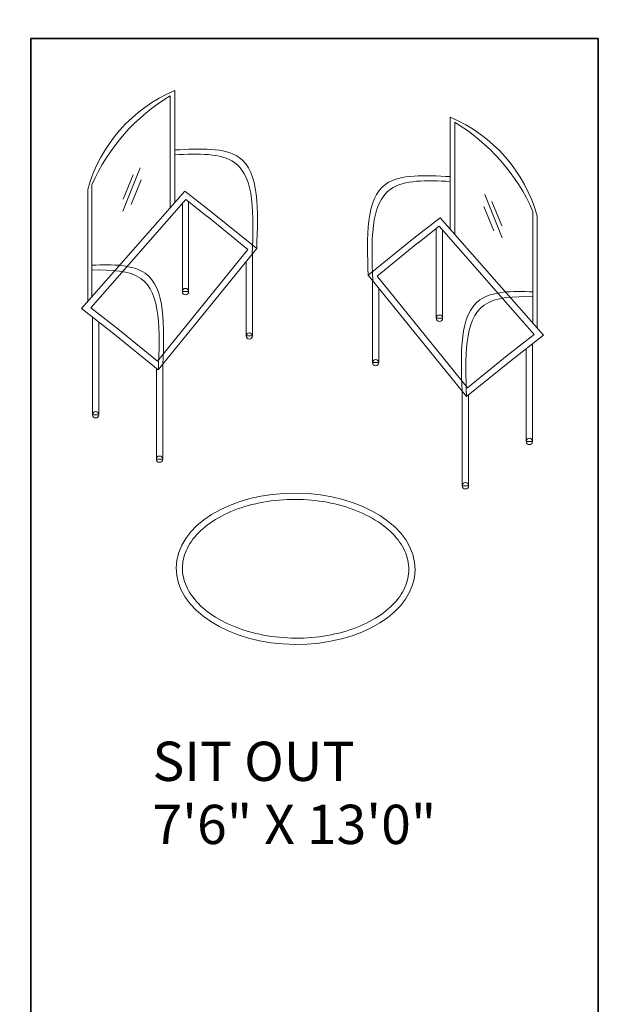
# Model space of a CAD drawing. Units: inches. Extents: x -61 to 1599, y -1316 to 257.
# Tile 97 of 204: x 22 to 114, y -166 to -10. Entities that reach past the tile are written whole.
import ezdxf

# ---------------------------------------------------------------- set-up
doc = ezdxf.new("R2010")
doc.units = ezdxf.units.IN
doc.header["$MEASUREMENT"] = 0
for name, color, linetype, lineweight in [('A-ANNO-DIMS', 2, 'Continuous', 18), ('A-AREA-IDEN', 1, 'Continuous', 18), ('FURNITURE', 83, 'Continuous', 18), ('WALLS', 4, 'Continuous', 35)]:
    doc.layers.add(name, color=color, linetype=linetype, lineweight=lineweight)
doc.styles.get("Standard").update_dxf_attribs({"font": 'arial.ttf'})
doc.dimstyles.get("Standard").update_dxf_attribs({"dimtxt": 0.18, "dimasz": 0.18, "dimexe": 0.18, "dimexo": 0.0625, "dimgap": 0.09, "dimtad": 0, "dimtih": 1, "dimtoh": 1, "dimdec": 0, "dimzin": 0, "dimdsep": 46, "dimlunit": 3, "dimtxsty": 'Standard', "dimcen": 0.09, "dimadec": 0, "dimazin": 0, "dimtfac": 1, "dimtdec": 0, "dimtofl": 0, "dimtmove": 0, "dimatfit": 3, "dimfxl": 1, "dimtolj": 1, "dimtzin": 0, "dimarcsym": 0})

# ---------------------------------------------------------------- blocks, each defined once
blk = doc.blocks.new('LOUNGE-CHAIR')
for p, q in [((14.04, 40.33), (14.04, 58.08)), ((14.76, 41.14), (14.76, 58.89)), ((6.52, 39.78), (9.29, 46.65)), ((6.58, 41.68), (8.18, 45.54)), ((1.64, 26.22), (1.64, 43.97)), ((7.84, 40.87), (9.45, 44.74)), ((0, 24.35), (16.38, 42.98)), ((0.97, 25.45), (0.97, 43.2)), ((0.97, 25.45), (0.97, 43.2)), ((16.38, 42.98), (20.51, 39.74)), ((16.97, 42.52), (16.97, 42.52)), ((1.45, 24.49), (16.5, 41.61)), ((15.97, 27.05), (15.97, 41.01)), ((16.5, 41.61), (19.89, 38.96)), ((16.97, 27.05), (16.97, 41.25)), ((20.51, 39.74), (27.76, 33.87)), ((19.88, 38.97), (26.35, 33.72)), ((12.02, 16.03), (26.35, 33.72)), ((12.16, 14.63), (27.76, 33.87)), ((27.1, 20.02), (27.1, 33.05)), ((26.1, 20.02), (26.1, 31.82)), ((16.97, 27.05), (15.97, 27.05)), ((0, 24.35), (5.1, 20.35)), ((0.75, 23.69), (0.79, 23.74)), ((1.45, 24.49), (5.72, 21.14)), ((1.73, 7.53), (1.73, 23)), ((2.73, 7.53), (2.73, 22.21)), ((5.1, 20.35), (12.16, 14.63)), ((5.73, 21.13), (12.02, 16.03)), ((27.1, 20.02), (26.1, 20.02)), ((11.85, 0.5), (11.85, 14.88)), ((12.85, 0.5), (12.85, 15.48)), ((2.73, 7.53), (1.73, 7.53)), ((12.85, 0.5), (11.85, 0.5))]:
    blk.add_line(p, q)
for centre in [(16.47, 27.05), (26.6, 20.02), (2.23, 7.53), (12.35, 0.5)]:
    blk.add_circle(centre, 0.5)
for centre, radius, start, end in [((23.93, 36.92), 23.8, 112.6586, 164.6996), ((30.25, 31.33), 31.28, 121.203, 156.1552)]:
    blk.add_arc(centre, radius, start, end)
for points, knots in [([(14.76, 49.49), (18.73, 49.7), (28.38, 50.23), (27.99, 39.93), (27.76, 33.87)], [0, 0, 0, 0, 10.281855, 24.983674, 24.983674, 24.983674, 24.983674]), ([(14.76, 48.72), (18.48, 48.91), (27.65, 49.16), (27.27, 39.12), (27.05, 33.06), (27.04, 33.03), (27.04, 33.01), (27.04, 32.98)], [0.614676, 0.614676, 0.614676, 0.614676, 10.281855, 24.983674, 24.983674, 24.983674, 25.041855, 25.041855, 25.041855, 25.041855]), ([(1.64, 31.22), (4.99, 31.37), (13.47, 31.24), (13.11, 21.57), (12.88, 15.51)], [1.527723, 1.527723, 1.527723, 1.527723, 10.281855, 24.983674, 24.983674, 24.983674, 24.983674]), ([(1.64, 30.44), (4.72, 30.55), (12.75, 30.17), (12.39, 20.76), (12.17, 14.7), (12.16, 14.67), (12.16, 14.65), (12.16, 14.63)], [2.150702, 2.150702, 2.150702, 2.150702, 10.281855, 24.983674, 24.983674, 24.983674, 25.041855, 25.041855, 25.041855, 25.041855])]:
    blk.add_open_spline(points, degree=3, knots=knots)
blk = doc.blocks.new('SIDE-TABLE-OVAL')
blk.add_ellipse((18.95, 11.99), major_axis=(-18.95, 0.16), ratio=0.632617)
blk.add_open_spline([(1, 12.14), (0.99, 11.17), (1.2, 10.2), (2.05, 8.28), (2.69, 7.34), (4.41, 5.58), (5.48, 4.76), (7.96, 3.32), (9.37, 2.71), (12.41, 1.74), (14.05, 1.4), (17.41, 1), (19.13, 0.95), (22.53, 1.15), (24.2, 1.41), (27.36, 2.19), (28.84, 2.73), (31.49, 4.02), (32.66, 4.78), (34.59, 6.45), (35.35, 7.36), (36.44, 9.24), (36.76, 10.2), (36.97, 12.14), (36.87, 13.11), (36.22, 15.04), (35.67, 16), (34.15, 17.81), (33.17, 18.67), (30.85, 20.19), (29.51, 20.86), (26.58, 21.94), (24.98, 22.36), (21.67, 22.89), (19.95, 23.01), (16.54, 22.94), (14.84, 22.76), (11.61, 22.1), (10.07, 21.63), (7.28, 20.44), (6.03, 19.73), (3.92, 18.13), (3.06, 17.25), (1.78, 15.4), (1.35, 14.44), (1.05, 13.03), (1, 12.59), (1, 12.14)], degree=3, knots=[0, 0, 0, 0, 0.279765, 0.279765, 0.559529, 0.559529, 0.839294, 0.839294, 1.119059, 1.119059, 1.398823, 1.398823, 1.678588, 1.678588, 1.958353, 1.958353, 2.238118, 2.238118, 2.517882, 2.517882, 2.797647, 2.797647, 3.077412, 3.077412, 3.357176, 3.357176, 3.636941, 3.636941, 3.916706, 3.916706, 4.19647, 4.19647, 4.476235, 4.476235, 4.756, 4.756, 5.035764, 5.035764, 5.315529, 5.315529, 5.595294, 5.595294, 5.875058, 5.875058, 6.154823, 6.154823, 6.283185, 6.283185, 6.283185, 6.283185])
blk = doc.blocks.new('*D687')
at = {"layer": 'A-ANNO-DIMS', "color": 0, "lineweight": -2, "transparency": 16777216}
for p, q in [((289.42, 181.68), (-61.08, 181.68)), ((-60.9, 181.5), (-60.9, -528.95)), ((-60.9, -1239.76), (-60.9, -529.32)), ((319.64, -1239.94), (-61.08, -1239.94))]:
    blk.add_line(p, q, dxfattribs=at)
at = {"layer": 'A-ANNO-DIMS', "color": 0, "transparency": 16777216}
for points in [[(-60.93, 181.5), (-60.87, 181.5), (-60.9, 181.68)], [(-60.93, -1239.76), (-60.87, -1239.76), (-60.9, -1239.94)]]:
    blk.add_solid(points, dxfattribs=at)
at = {"layer": 'DEFPOINTS', "color": 0, "transparency": 16777216}
for p in [(289.48, 181.68), (-60.9, -1239.94), (319.7, -1239.94)]:
    blk.add_point(p, dxfattribs=at)
at = {"layer": 'A-ANNO-DIMS', "color": 0, "transparency": 16777216, "insert": (-60.9, -529.13), "char_height": 0.18, "attachment_point": 5}
blk.add_mtext('\\A1;1421.6', dxfattribs=at)
blk = doc.blocks.new('*D700')
at = {"layer": 'A-ANNO-DIMS', "color": 0, "lineweight": -2, "transparency": 16777216}
for p, q in [((14.7, -616.88), (14.7, 257.46)), ((179.75, -616.88), (179.75, 257.46)), ((14.88, 257.28), (96.77, 257.28)), ((179.57, 257.28), (97.68, 257.28))]:
    blk.add_line(p, q, dxfattribs=at)
at = {"layer": 'A-ANNO-DIMS', "color": 0, "transparency": 16777216}
for points in [[(14.88, 257.31), (14.88, 257.25), (14.7, 257.28)], [(179.57, 257.31), (179.57, 257.25), (179.75, 257.28)]]:
    blk.add_solid(points, dxfattribs=at)
at = {"layer": 'DEFPOINTS', "color": 0, "transparency": 16777216}
for p in [(179.75, 257.28), (14.7, -616.94), (179.75, -616.94)]:
    blk.add_point(p, dxfattribs=at)
at = {"layer": 'A-ANNO-DIMS', "color": 0, "transparency": 16777216, "insert": (97.23, 257.28), "char_height": 0.18, "attachment_point": 5}
blk.add_mtext('\\A1;165.05', dxfattribs=at)

msp = doc.modelspace()

# ---------------------------------------------------------------- linework, layer by layer
at = {"layer": 'WALLS'}
for p, q in [((23.7028, -13.3229), (113.7028, -13.3229)), ((23.7028, -169.3229), (23.7028, -13.3229)), ((113.7028, -169.3229), (113.7028, -13.3229))]:
    msp.add_line(p, q, dxfattribs=at)

# ---------------------------------------------------------------- block references
at = {"layer": 'FURNITURE'}
for name, p in [('LOUNGE-CHAIR', (31.776, -80.445)), ('SIDE-TABLE-OVAL', (46.761, -109.297))]:
    msp.add_blockref(name, p, dxfattribs=at)
at = {"layer": 'FURNITURE', "extrusion": (0, 0, -1), "zscale": -1}
msp.add_blockref('LOUNGE-CHAIR', (-104.9843, -84.6679), dxfattribs=at)

# ---------------------------------------------------------------- texts
at = {"layer": 'A-AREA-IDEN'}
for s, height, p in [('SIT OUT', 6.22364, (43.0043, -130.923)), ('7\'6" X 13\'0"', 6.223643, (43.0043, -140.9207))]:
    msp.add_text(s, height=height, dxfattribs=at).set_placement(p)

# ---------------------------------------------------------------- dimensions: what is measured, and where the dimension line sits
at = {"layer": 'A-ANNO-DIMS'}
dim = msp.add_linear_dim(base=(179.7521, 257.2771), p1=(14.7028, -616.9446), p2=(179.7521, -616.9446), dimstyle='Standard', override={"dimdec": 2, "dimlfac": 1, "dimrnd": 0, "dimzin": 0, "dimdsep": 46, "dimlunit": 2}, dxfattribs=at)
dim.commit()
dim.dimension.update_dxf_attribs({"geometry": '*D700', "text_midpoint": (97.2274, 257.2771)})
dim = msp.add_linear_dim(base=(-60.8972, -1239.9446), p1=(289.4807, 181.6771), p2=(319.7028, -1239.9446), angle=90, dimstyle='Standard', override={"dimdec": 1, "dimlfac": 1, "dimrnd": 0, "dimzin": 0, "dimdsep": 46, "dimlunit": 2}, dxfattribs=at)
dim.commit()
dim.dimension.update_dxf_attribs({"geometry": '*D687', "text_midpoint": (-60.8972, -529.1337)})

doc.saveas('drawing.dxf')
